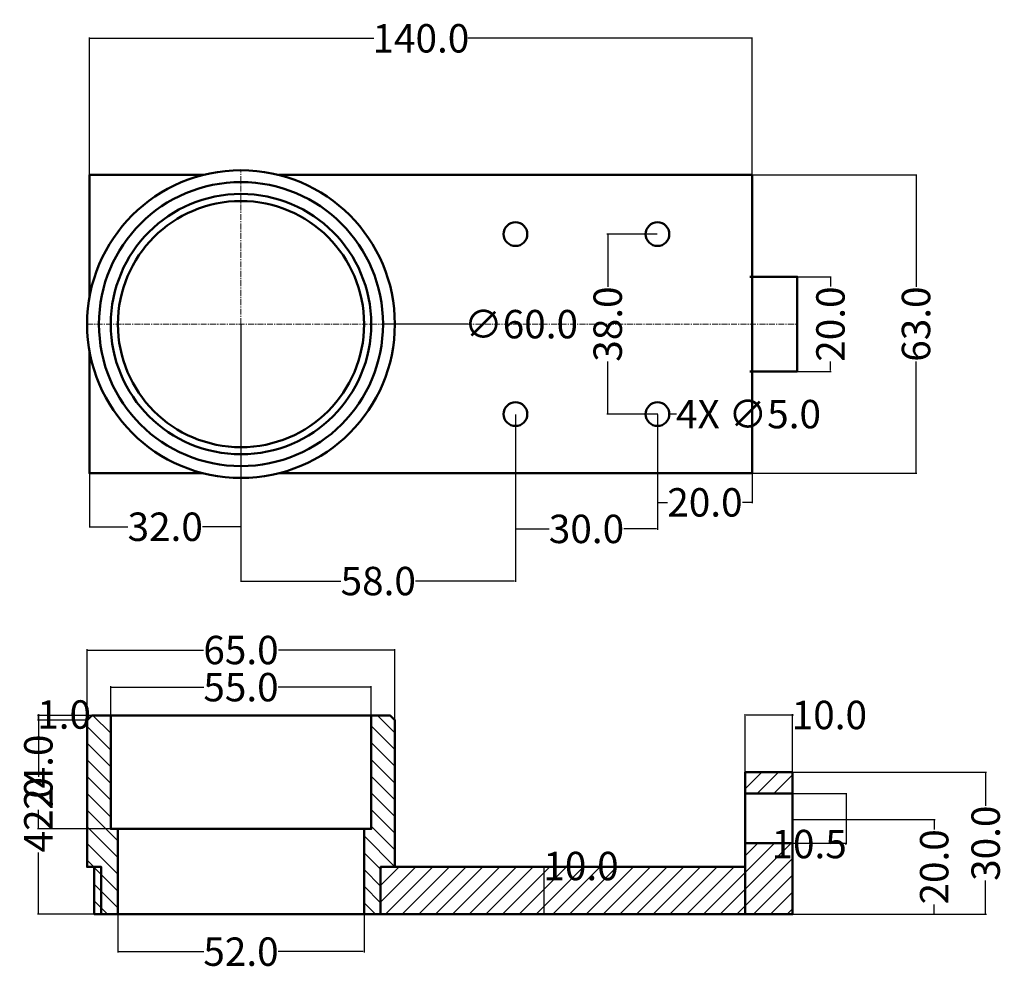
# Model space of a CAD drawing. Units: millimetres. Extents: x 92 to 300, y 40 to 241.
import ezdxf

# ---------------------------------------------------------------- set-up
doc = ezdxf.new("R2010")
doc.units = ezdxf.units.MM
doc.header["$MEASUREMENT"] = 0
doc.linetypes.add('CENTER', pattern=[2, 1.25, -0.25, 0.25, -0.25])
for name, color, linetype, lineweight in [('M-CNTR', 1, 'CENTER', 18), ('M-CONS', 8, 'Continuous', 13), ('M-DIMS', 2, 'Continuous', 25), ('M-HATC', 8, 'Continuous', 18), ('M-OUTL', 7, 'Continuous', 50), ('M-TEXT', 3, 'Continuous', 25)]:
    doc.layers.add(name, color=color, linetype=linetype, lineweight=lineweight)
doc.styles.get("Standard").update_dxf_attribs({"font": 'arial.ttf'})
doc.dimstyles.get("Standard").update_dxf_attribs({"dimtxt": 6, "dimasz": 0.18, "dimexe": 0.18, "dimexo": 0.0625, "dimgap": 0.09, "dimtad": 0, "dimtoh": 1, "dimdec": 1, "dimzin": 0, "dimdsep": 46, "dimtxsty": 'Standard', "dimcen": 0.09, "dimadec": 0, "dimazin": 0, "dimtfac": 1, "dimtdec": 1, "dimtofl": 0, "dimtmove": 0, "dimatfit": 3, "dimfxl": 1, "dimtolj": 1, "dimtzin": 0, "dimarcsym": 0})
pattern_1 = [(45, (89.012, 127.1657), (-1.767767, 1.767767), [])]

# ---------------------------------------------------------------- blocks, each defined once
blk = doc.blocks.new('*D1')
at = {"layer": 'Defpoints', "color": 0, "transparency": 16777216}
for p in [(247.12, 208.35), (247.12, 145.35), (281.69, 145.35)]:
    blk.add_point(p, dxfattribs=at)
at = {"layer": 'M-DIMS', "color": 0, "lineweight": -2, "transparency": 16777216}
for p, q in [((247.18, 208.35), (281.87, 208.35)), ((281.69, 208.17), (281.69, 184.73)), ((281.69, 145.53), (281.69, 168.96)), ((247.18, 145.35), (281.87, 145.35))]:
    blk.add_line(p, q, dxfattribs=at)
at = {"layer": 'M-DIMS', "color": 0, "transparency": 16777216}
for points in [[(281.66, 208.17), (281.72, 208.17), (281.69, 208.35)], [(281.66, 145.53), (281.72, 145.53), (281.69, 145.35)]]:
    blk.add_solid(points, dxfattribs=at)
at = {"layer": 'M-DIMS', "color": 0, "transparency": 16777216, "insert": (281.69, 176.85), "char_height": 6, "attachment_point": 5, "rotation": 90}
blk.add_mtext('\\A1;63.0', dxfattribs=at)
blk = doc.blocks.new('*D2')
at = {"layer": 'Defpoints', "color": 0, "transparency": 16777216}
for p in [(256.62, 186.85), (256.62, 166.85), (263.62, 166.85)]:
    blk.add_point(p, dxfattribs=at)
at = {"layer": 'M-DIMS', "color": 0, "lineweight": -2, "transparency": 16777216}
for p, q in [((256.68, 186.85), (263.8, 186.85)), ((263.62, 186.67), (263.62, 184.77)), ((263.62, 167.03), (263.62, 168.92)), ((256.68, 166.85), (263.8, 166.85))]:
    blk.add_line(p, q, dxfattribs=at)
at = {"layer": 'M-DIMS', "color": 0, "transparency": 16777216}
for points in [[(263.59, 186.67), (263.65, 186.67), (263.62, 186.85)], [(263.59, 167.03), (263.65, 167.03), (263.62, 166.85)]]:
    blk.add_solid(points, dxfattribs=at)
at = {"layer": 'M-DIMS', "color": 0, "transparency": 16777216, "insert": (263.62, 176.85), "char_height": 6, "attachment_point": 5, "rotation": 90}
blk.add_mtext('\\A1;20.0', dxfattribs=at)
blk = doc.blocks.new('*D3')
at = {"layer": 'Defpoints', "color": 0, "transparency": 16777216}
for p in [(227.09, 195.85), (216.57, 157.85), (227.09, 157.85)]:
    blk.add_point(p, dxfattribs=at)
at = {"layer": 'M-DIMS', "color": 0, "lineweight": -2, "transparency": 16777216}
for p, q in [((227.03, 195.85), (216.39, 195.85)), ((216.57, 195.67), (216.57, 184.72)), ((216.57, 158.03), (216.57, 168.97)), ((227.03, 157.85), (216.39, 157.85))]:
    blk.add_line(p, q, dxfattribs=at)
at = {"layer": 'M-DIMS', "color": 0, "transparency": 16777216}
for points in [[(216.54, 195.67), (216.6, 195.67), (216.57, 195.85)], [(216.54, 158.03), (216.6, 158.03), (216.57, 157.85)]]:
    blk.add_solid(points, dxfattribs=at)
at = {"layer": 'M-DIMS', "color": 0, "transparency": 16777216, "insert": (216.57, 176.85), "char_height": 6, "attachment_point": 5, "rotation": 90}
blk.add_mtext('\\A1;38.0', dxfattribs=at)
blk = doc.blocks.new('*D4')
at = {"layer": 'Defpoints', "color": 0, "transparency": 16777216}
for p in [(107.12, 145.35), (139.12, 144.35), (107.12, 134.05)]:
    blk.add_point(p, dxfattribs=at)
at = {"layer": 'M-DIMS', "color": 0, "lineweight": -2, "transparency": 16777216}
for p, q in [((107.12, 145.28), (107.12, 133.87)), ((139.12, 144.28), (139.12, 133.87)), ((107.3, 134.05), (115.25, 134.05)), ((138.94, 134.05), (130.99, 134.05))]:
    blk.add_line(p, q, dxfattribs=at)
at = {"layer": 'M-DIMS', "color": 0, "transparency": 16777216}
for points in [[(107.3, 134.08), (107.3, 134.02), (107.12, 134.05)], [(138.94, 134.08), (138.94, 134.02), (139.12, 134.05)]]:
    blk.add_solid(points, dxfattribs=at)
at = {"layer": 'M-DIMS', "color": 0, "transparency": 16777216, "insert": (123.12, 134.05), "char_height": 6, "attachment_point": 5}
blk.add_mtext('\\A1;32.0', dxfattribs=at)
blk = doc.blocks.new('*D5')
at = {"layer": 'Defpoints', "color": 0, "transparency": 16777216}
for p in [(247.12, 237.21), (107.12, 208.35), (247.12, 208.35)]:
    blk.add_point(p, dxfattribs=at)
at = {"layer": 'M-DIMS', "color": 0, "lineweight": -2, "transparency": 16777216}
for p, q in [((107.12, 208.41), (107.12, 237.39)), ((107.3, 237.21), (167.2, 237.21)), ((246.94, 237.21), (187.04, 237.21)), ((247.12, 208.41), (247.12, 237.39))]:
    blk.add_line(p, q, dxfattribs=at)
at = {"layer": 'M-DIMS', "color": 0, "transparency": 16777216}
for points in [[(107.3, 237.24), (107.3, 237.18), (107.12, 237.21)], [(246.94, 237.24), (246.94, 237.18), (247.12, 237.21)]]:
    blk.add_solid(points, dxfattribs=at)
at = {"layer": 'M-DIMS', "color": 0, "transparency": 16777216, "insert": (177.12, 237.21), "char_height": 6, "attachment_point": 5}
blk.add_mtext('\\A1;140.0', dxfattribs=at)
blk = doc.blocks.new('*D6')
at = {"layer": 'Defpoints', "color": 0, "transparency": 16777216}
for p in [(197.09, 157.85), (227.09, 157.85), (227.09, 133.59)]:
    blk.add_point(p, dxfattribs=at)
at = {"layer": 'M-DIMS', "color": 0, "lineweight": -2, "transparency": 16777216}
for p, q in [((197.09, 157.78), (197.09, 133.41)), ((227.09, 157.78), (227.09, 133.41)), ((197.27, 133.59), (204.22, 133.59)), ((226.91, 133.59), (219.96, 133.59))]:
    blk.add_line(p, q, dxfattribs=at)
at = {"layer": 'M-DIMS', "color": 0, "transparency": 16777216}
for points in [[(197.27, 133.62), (197.27, 133.56), (197.09, 133.59)], [(226.91, 133.62), (226.91, 133.56), (227.09, 133.59)]]:
    blk.add_solid(points, dxfattribs=at)
at = {"layer": 'M-DIMS', "color": 0, "transparency": 16777216, "insert": (212.09, 133.59), "char_height": 6, "attachment_point": 5}
blk.add_mtext('\\A1;30.0', dxfattribs=at)
blk = doc.blocks.new('*D7')
at = {"layer": 'Defpoints', "color": 0, "transparency": 16777216}
for p in [(227.09, 145.35), (247.12, 145.35), (247.12, 139.2)]:
    blk.add_point(p, dxfattribs=at)
at = {"layer": 'M-DIMS', "color": 0, "lineweight": -2, "transparency": 16777216}
for p, q in [((227.09, 145.28), (227.09, 139.02)), ((247.12, 145.28), (247.12, 139.02)), ((227.27, 139.2), (229.18, 139.2)), ((246.94, 139.2), (245.03, 139.2))]:
    blk.add_line(p, q, dxfattribs=at)
at = {"layer": 'M-DIMS', "color": 0, "transparency": 16777216}
for points in [[(227.27, 139.23), (227.27, 139.17), (227.09, 139.2)], [(246.94, 139.23), (246.94, 139.17), (247.12, 139.2)]]:
    blk.add_solid(points, dxfattribs=at)
at = {"layer": 'M-DIMS', "color": 0, "transparency": 16777216, "insert": (237.11, 139.2), "char_height": 6, "attachment_point": 5}
blk.add_mtext('\\A1;20.0', dxfattribs=at)
blk = doc.blocks.new('*D8')
at = {"layer": 'Defpoints', "color": 0, "transparency": 16777216}
for p in [(139.12, 176.85), (197.09, 157.85), (197.09, 122.58)]:
    blk.add_point(p, dxfattribs=at)
at = {"layer": 'M-DIMS', "color": 0, "lineweight": -2, "transparency": 16777216}
for p, q in [((139.12, 176.78), (139.12, 122.4)), ((197.09, 157.78), (197.09, 122.4)), ((139.3, 122.58), (160.23, 122.58)), ((196.91, 122.58), (175.98, 122.58))]:
    blk.add_line(p, q, dxfattribs=at)
at = {"layer": 'M-DIMS', "color": 0, "transparency": 16777216}
for points in [[(139.3, 122.61), (139.3, 122.55), (139.12, 122.58)], [(196.91, 122.61), (196.91, 122.55), (197.09, 122.58)]]:
    blk.add_solid(points, dxfattribs=at)
at = {"layer": 'M-DIMS', "color": 0, "transparency": 16777216, "insert": (168.11, 122.58), "char_height": 6, "attachment_point": 5}
blk.add_mtext('\\A1;58.0', dxfattribs=at)
blk = doc.blocks.new('*D9')
at = {"layer": 'Defpoints', "color": 0, "transparency": 16777216}
for p in [(255.62, 72.21), (285.53, 72.21), (255.62, 52.21)]:
    blk.add_point(p, dxfattribs=at)
at = {"layer": 'M-DIMS', "color": 0, "lineweight": -2, "transparency": 16777216}
for p, q in [((255.68, 72.21), (285.71, 72.21)), ((285.53, 72.03), (285.53, 70.13)), ((285.53, 52.39), (285.53, 54.29)), ((255.68, 52.21), (285.71, 52.21))]:
    blk.add_line(p, q, dxfattribs=at)
at = {"layer": 'M-DIMS', "color": 0, "transparency": 16777216}
for points in [[(285.5, 72.03), (285.56, 72.03), (285.53, 72.21)], [(285.5, 52.39), (285.56, 52.39), (285.53, 52.21)]]:
    blk.add_solid(points, dxfattribs=at)
at = {"layer": 'M-DIMS', "color": 0, "transparency": 16777216, "insert": (285.53, 62.21), "char_height": 6, "attachment_point": 5, "rotation": 90}
blk.add_mtext('\\A1;20.0', dxfattribs=at)
blk = doc.blocks.new('*D10')
at = {"layer": 'Defpoints', "color": 0, "transparency": 16777216}
for p in [(255.62, 94.29), (245.62, 82.21), (255.62, 82.21)]:
    blk.add_point(p, dxfattribs=at)
at = {"layer": 'M-DIMS', "color": 0, "lineweight": -2, "transparency": 16777216}
for p, q in [((245.62, 82.27), (245.62, 94.47)), ((245.8, 94.29), (255.44, 94.29)), ((255.62, 82.27), (255.62, 94.47)), ((255.62, 94.29), (255.8, 94.29))]:
    blk.add_line(p, q, dxfattribs=at)
at = {"layer": 'M-DIMS', "color": 0, "transparency": 16777216}
for points in [[(245.8, 94.32), (245.8, 94.26), (245.62, 94.29)], [(255.44, 94.32), (255.44, 94.26), (255.62, 94.29)]]:
    blk.add_solid(points, dxfattribs=at)
at = {"layer": 'M-DIMS', "color": 0, "transparency": 16777216, "insert": (263.39, 94.29), "char_height": 6, "attachment_point": 5}
blk.add_mtext('\\A1;10.0', dxfattribs=at)
blk = doc.blocks.new('*D11')
at = {"layer": 'Defpoints', "color": 0, "transparency": 16777216}
for p in [(166.62, 100.17), (111.62, 94.21), (166.62, 94.21)]:
    blk.add_point(p, dxfattribs=at)
at = {"layer": 'M-DIMS', "color": 0, "lineweight": -2, "transparency": 16777216}
for p, q in [((111.62, 94.27), (111.62, 100.35)), ((111.8, 100.17), (131.25, 100.17)), ((166.44, 100.17), (146.99, 100.17)), ((166.62, 94.27), (166.62, 100.35))]:
    blk.add_line(p, q, dxfattribs=at)
at = {"layer": 'M-DIMS', "color": 0, "transparency": 16777216}
for points in [[(111.8, 100.2), (111.8, 100.14), (111.62, 100.17)], [(166.44, 100.2), (166.44, 100.14), (166.62, 100.17)]]:
    blk.add_solid(points, dxfattribs=at)
at = {"layer": 'M-DIMS', "color": 0, "transparency": 16777216, "insert": (139.12, 100.17), "char_height": 6, "attachment_point": 5}
blk.add_mtext('\\A1;55.0', dxfattribs=at)
blk = doc.blocks.new('*D12')
at = {"layer": 'Defpoints', "color": 0, "transparency": 16777216}
for p in [(171.62, 108.01), (106.62, 93.21), (171.62, 93.21)]:
    blk.add_point(p, dxfattribs=at)
at = {"layer": 'M-DIMS', "color": 0, "lineweight": -2, "transparency": 16777216}
for p, q in [((106.62, 93.27), (106.62, 108.19)), ((171.62, 93.27), (171.62, 108.19)), ((106.8, 108.01), (131.23, 108.01)), ((171.44, 108.01), (147.01, 108.01))]:
    blk.add_line(p, q, dxfattribs=at)
at = {"layer": 'M-DIMS', "color": 0, "transparency": 16777216}
for points in [[(106.8, 108.04), (106.8, 107.98), (106.62, 108.01)], [(171.44, 108.04), (171.44, 107.98), (171.62, 108.01)]]:
    blk.add_solid(points, dxfattribs=at)
at = {"layer": 'M-DIMS', "color": 0, "transparency": 16777216, "insert": (139.12, 108.01), "char_height": 6, "attachment_point": 5}
blk.add_mtext('\\A1;65.0', dxfattribs=at)
blk = doc.blocks.new('*D13')
at = {"layer": 'Defpoints', "color": 0, "transparency": 16777216}
for p in [(113.12, 52.21), (165.12, 52.21), (165.12, 44.3)]:
    blk.add_point(p, dxfattribs=at)
at = {"layer": 'M-DIMS', "color": 0, "lineweight": -2, "transparency": 16777216}
for p, q in [((113.12, 52.15), (113.12, 44.12)), ((165.12, 52.15), (165.12, 44.12)), ((113.3, 44.3), (131.25, 44.3)), ((164.94, 44.3), (146.99, 44.3))]:
    blk.add_line(p, q, dxfattribs=at)
at = {"layer": 'M-DIMS', "color": 0, "transparency": 16777216}
for points in [[(113.3, 44.33), (113.3, 44.27), (113.12, 44.3)], [(164.94, 44.33), (164.94, 44.27), (165.12, 44.3)]]:
    blk.add_solid(points, dxfattribs=at)
at = {"layer": 'M-DIMS', "color": 0, "transparency": 16777216, "insert": (139.12, 44.3), "char_height": 6, "attachment_point": 5}
blk.add_mtext('\\A1;52.0', dxfattribs=at)
blk = doc.blocks.new('*D14')
at = {"layer": 'Defpoints', "color": 0, "transparency": 16777216}
for p in [(203.16, 62.21), (207.12, 62.21), (207.12, 52.21)]:
    blk.add_point(p, dxfattribs=at)
at = {"layer": 'M-DIMS', "color": 0, "lineweight": -2, "transparency": 16777216}
for p, q in [((203.16, 62.21), (203.16, 62.39)), ((203.16, 62.39), (203.34, 62.39)), ((207.06, 62.21), (202.98, 62.21)), ((203.16, 52.39), (203.16, 62.03)), ((207.06, 52.21), (202.98, 52.21))]:
    blk.add_line(p, q, dxfattribs=at)
at = {"layer": 'M-DIMS', "color": 0, "transparency": 16777216}
for points in [[(203.13, 62.03), (203.19, 62.03), (203.16, 62.21)], [(203.13, 52.39), (203.19, 52.39), (203.16, 52.21)]]:
    blk.add_solid(points, dxfattribs=at)
at = {"layer": 'M-DIMS', "color": 0, "transparency": 16777216, "insert": (210.93, 62.39), "char_height": 6, "attachment_point": 5}
blk.add_mtext('\\A1;10.0', dxfattribs=at)
blk = doc.blocks.new('*D15')
at = {"layer": 'Defpoints', "color": 0, "transparency": 16777216}
for p in [(250.62, 82.21), (250.62, 52.21), (296.4, 52.21)]:
    blk.add_point(p, dxfattribs=at)
at = {"layer": 'M-DIMS', "color": 0, "lineweight": -2, "transparency": 16777216}
for p, q in [((250.68, 82.21), (296.58, 82.21)), ((296.4, 82.03), (296.4, 75.08)), ((296.4, 52.39), (296.4, 59.34)), ((250.68, 52.21), (296.58, 52.21))]:
    blk.add_line(p, q, dxfattribs=at)
at = {"layer": 'M-DIMS', "color": 0, "transparency": 16777216}
for points in [[(296.37, 82.03), (296.43, 82.03), (296.4, 82.21)], [(296.37, 52.39), (296.43, 52.39), (296.4, 52.21)]]:
    blk.add_solid(points, dxfattribs=at)
at = {"layer": 'M-DIMS', "color": 0, "transparency": 16777216, "insert": (296.4, 67.21), "char_height": 6, "attachment_point": 5, "rotation": 90}
blk.add_mtext('\\A1;30.0', dxfattribs=at)
blk = doc.blocks.new('HOLE-M5')
blk.add_circle((2.5, 2.5), 2.5)
blk = doc.blocks.new('*D17')
at = {"layer": 'Defpoints', "color": 0, "transparency": 16777216}
for p in [(107.62, 94.21), (96.32, 52.21), (108.12, 52.21)]:
    blk.add_point(p, dxfattribs=at)
at = {"layer": 'M-DIMS', "color": 0, "lineweight": -2, "transparency": 16777216}
for p, q in [((107.56, 94.21), (96.14, 94.21)), ((96.32, 94.03), (96.32, 81.2)), ((96.32, 52.39), (96.32, 65.22)), ((108.06, 52.21), (96.14, 52.21))]:
    blk.add_line(p, q, dxfattribs=at)
at = {"layer": 'M-DIMS', "color": 0, "transparency": 16777216}
for points in [[(96.29, 94.03), (96.35, 94.03), (96.32, 94.21)], [(96.29, 52.39), (96.35, 52.39), (96.32, 52.21)]]:
    blk.add_solid(points, dxfattribs=at)
at = {"layer": 'M-DIMS', "color": 0, "transparency": 16777216, "insert": (96.32, 73.21), "char_height": 6, "attachment_point": 5, "rotation": 90}
blk.add_mtext('\\A1;42.0', dxfattribs=at)
blk = doc.blocks.new('*D18')
at = {"layer": 'Defpoints', "color": 0, "transparency": 16777216}
for p in [(111.62, 94.21), (96.32, 70.21), (111.62, 70.21)]:
    blk.add_point(p, dxfattribs=at)
at = {"layer": 'M-DIMS', "color": 0, "lineweight": -2, "transparency": 16777216}
for p, q in [((111.56, 94.21), (96.14, 94.21)), ((96.32, 94.03), (96.32, 90.13)), ((96.32, 70.39), (96.32, 74.29)), ((111.56, 70.21), (96.14, 70.21))]:
    blk.add_line(p, q, dxfattribs=at)
at = {"layer": 'M-DIMS', "color": 0, "transparency": 16777216}
for points in [[(96.29, 94.03), (96.35, 94.03), (96.32, 94.21)], [(96.29, 70.39), (96.35, 70.39), (96.32, 70.21)]]:
    blk.add_solid(points, dxfattribs=at)
at = {"layer": 'M-DIMS', "color": 0, "transparency": 16777216, "insert": (96.32, 82.21), "char_height": 6, "attachment_point": 5, "rotation": 90}
blk.add_mtext('\\A1;24.0', dxfattribs=at)
blk = doc.blocks.new('*D19')
at = {"layer": 'Defpoints', "color": 0, "transparency": 16777216}
for p in [(96.32, 94.21), (107.62, 94.21), (106.62, 93.21)]:
    blk.add_point(p, dxfattribs=at)
at = {"layer": 'M-DIMS', "color": 0, "lineweight": -2, "transparency": 16777216}
for p, q in [((107.56, 94.21), (96.14, 94.21)), ((96.32, 94.21), (96.32, 94.39)), ((96.32, 94.39), (96.5, 94.39)), ((96.32, 93.39), (96.32, 94.03)), ((106.56, 93.21), (96.14, 93.21))]:
    blk.add_line(p, q, dxfattribs=at)
at = {"layer": 'M-DIMS', "color": 0, "transparency": 16777216}
for points in [[(96.29, 94.03), (96.35, 94.03), (96.32, 94.21)], [(96.29, 93.39), (96.35, 93.39), (96.32, 93.21)]]:
    blk.add_solid(points, dxfattribs=at)
at = {"layer": 'M-DIMS', "color": 0, "transparency": 16777216, "insert": (101.76, 94.39), "char_height": 6, "attachment_point": 5}
blk.add_mtext('\\A1;1.0', dxfattribs=at)
blk = doc.blocks.new('*D20')
at = {"layer": 'Defpoints', "color": 0, "transparency": 16777216}
for p in [(255.62, 77.71), (255.62, 67.21), (266.92, 67.21)]:
    blk.add_point(p, dxfattribs=at)
at = {"layer": 'M-DIMS', "color": 0, "lineweight": -2, "transparency": 16777216}
for p, q in [((255.68, 77.71), (267.1, 77.71)), ((266.92, 77.53), (266.92, 67.39)), ((255.68, 67.21), (267.1, 67.21)), ((266.92, 67.03), (266.74, 67.03)), ((266.92, 67.21), (266.92, 67.03))]:
    blk.add_line(p, q, dxfattribs=at)
at = {"layer": 'M-DIMS', "color": 0, "transparency": 16777216}
for points in [[(266.89, 77.53), (266.95, 77.53), (266.92, 77.71)], [(266.89, 67.39), (266.95, 67.39), (266.92, 67.21)]]:
    blk.add_solid(points, dxfattribs=at)
at = {"layer": 'M-DIMS', "color": 0, "transparency": 16777216, "insert": (259.12, 67.03), "char_height": 6, "attachment_point": 5}
blk.add_mtext('\\A1;10.5', dxfattribs=at)
blk = doc.blocks.new('*D21')
at = {"layer": 'Defpoints', "color": 0, "transparency": 16777216}
for p in [(109.12, 176.85), (169.12, 176.84)]:
    blk.add_point(p, dxfattribs=at)
at = {"layer": 'M-DIMS', "color": 0, "lineweight": -2, "transparency": 16777216}
for p, q in [((139.03, 176.85), (139.21, 176.85)), ((139.12, 176.76), (139.12, 176.94)), ((187.12, 176.84), (169.3, 176.84))]:
    blk.add_line(p, q, dxfattribs=at)
at = {"layer": 'M-DIMS', "color": 0, "transparency": 16777216}
blk.add_solid([(169.3, 176.87), (169.3, 176.81), (169.12, 176.84)], dxfattribs=at)
at = {"layer": 'M-DIMS', "color": 0, "transparency": 16777216, "insert": (198.26, 176.84), "char_height": 6, "attachment_point": 5}
blk.add_mtext('\\A1;∅60.0', dxfattribs=at)
blk = doc.blocks.new('*D22')
at = {"layer": 'Defpoints', "color": 0, "transparency": 16777216}
for p in [(224.59, 157.85), (229.59, 157.84)]:
    blk.add_point(p, dxfattribs=at)
at = {"layer": 'M-DIMS', "color": 0, "lineweight": -2, "transparency": 16777216}
for p, q in [((227, 157.85), (227.18, 157.85)), ((227.09, 157.76), (227.09, 157.94)), ((231.09, 157.84), (229.77, 157.84))]:
    blk.add_line(p, q, dxfattribs=at)
at = {"layer": 'M-DIMS', "color": 0, "transparency": 16777216}
blk.add_solid([(229.77, 157.87), (229.77, 157.81), (229.59, 157.84)], dxfattribs=at)
at = {"layer": 'M-DIMS', "color": 0, "transparency": 16777216, "insert": (246.31, 157.84), "char_height": 6, "attachment_point": 5}
blk.add_mtext('\\A1;4X ∅5.0', dxfattribs=at)

msp = doc.modelspace()

# ---------------------------------------------------------------- hatches: boundary and pattern name
at = {"layer": 'M-HATC'}
h = msp.add_hatch(dxfattribs=at)
h.set_pattern_fill('ANSI31', color=256, scale=20, angle=90)
h.set_pattern_definition([(135, (89.012, 127.1657), (-1.767767, -1.767767), [])])
h.paths.add_polyline_path([(111.62, 94.21), (107.62, 94.21), (106.62, 93.21), (106.62, 62.21), (109.62, 62.21), (109.62, 52.21), (113.12, 52.21), (113.12, 70.21), (111.62, 70.21)])
h.paths.add_polyline_path([(171.62, 93.21), (170.62, 94.21), (166.62, 94.21), (166.62, 70.21), (165.12, 70.21), (165.12, 52.21), (168.62, 52.21), (168.62, 62.21), (171.62, 62.21)])
h.paths.add_polyline_path([(109.62, 62.21), (108.12, 62.21), (108.12, 52.21), (109.62, 52.21)], flags=17)
h = msp.add_hatch(dxfattribs=at)
h.set_pattern_fill('ANSI31', color=256, scale=20)
h.set_pattern_definition(pattern_1)
h.paths.add_polyline_path([(255.62, 77.71), (255.62, 82.21), (245.62, 82.21), (245.62, 77.71)])
h.paths.add_polyline_path([(245.62, 52.21), (255.62, 52.21), (255.62, 67.21), (245.62, 67.21), (245.62, 62.21)])
h = msp.add_hatch(dxfattribs=at)
h.set_pattern_fill('ANSI31', color=256, scale=20)
h.set_pattern_definition(pattern_1)
h.paths.add_polyline_path([(245.62, 52.21), (245.62, 62.21), (171.62, 62.21), (168.62, 62.21), (168.62, 52.21)])

# ---------------------------------------------------------------- linework, layer by layer
at = {"layer": 'M-CNTR'}
msp.add_line((108.2, 186.85), (108.12, 186.85), dxfattribs=at)
for points in [[(139.12, 144.35), (139.12, 150.85), (139.12, 202.85), (139.12, 209.35)], [(106.62, 176.85), (246.62, 176.85), (256.62, 176.85)]]:
    msp.add_lwpolyline(points, dxfattribs=at)
at = {"layer": 'M-CONS'}
msp.add_line((227.09, 145.35), (227.09, 157.85), dxfattribs=at)
at = {"layer": 'M-OUTL'}
for p, q in [((111.62, 94.21), (111.62, 70.21)), ((255.62, 77.71), (245.62, 77.71)), ((255.62, 67.21), (245.62, 67.21))]:
    msp.add_line(p, q, dxfattribs=at)
for points in [[(107.12, 182.52), (107.12, 208.35), (131.12, 208.35)], [(147.12, 145.35), (247.12, 145.35), (247.12, 208.35), (147.12, 208.35)], [(246.62, 186.85), (256.62, 186.85), (256.62, 166.85), (246.62, 166.85)], [(107.12, 171.17), (107.12, 145.35), (131.12, 145.35)], [(166.62, 94.21), (111.62, 94.21), (107.62, 94.21), (106.62, 93.21), (106.62, 62.21), (109.62, 62.21), (109.62, 52.21)], [(245.62, 62.21), (245.62, 52.21), (255.62, 52.21), (255.62, 82.21), (245.62, 82.21), (245.62, 62.21), (171.62, 62.21), (171.62, 93.21), (170.62, 94.21), (166.62, 94.21), (166.62, 70.21), (111.62, 70.21), (113.12, 70.21), (113.12, 52.21)], [(245.62, 52.21), (245.62, 52.21), (168.62, 52.21), (165.12, 52.21), (165.12, 70.21)], [(165.12, 52.21), (113.12, 52.21), (109.62, 52.21), (108.12, 52.21), (108.12, 62.21)], [(171.62, 62.21), (168.62, 62.21), (168.62, 52.21)]]:
    msp.add_lwpolyline(points, dxfattribs=at)
for radius in [32.5, 30, 27.5, 26]:
    msp.add_circle((139.12, 176.85), radius, dxfattribs=at)

# ---------------------------------------------------------------- block references
for p in [(194.59, 193.35), (224.59, 193.35), (194.59, 155.34), (224.59, 155.34)]:
    msp.add_blockref('HOLE-M5', p, dxfattribs=at)

# ---------------------------------------------------------------- texts
at = {"layer": 'M-TEXT'}
msp.add_attdef('M5', (199.57, 158.18), '', height=0.2, dxfattribs=at)

# ---------------------------------------------------------------- dimensions: what is measured, and where the dimension line sits
at = {"layer": 'M-DIMS'}
for base, p1, p2, picture, middle in [((247.12, 237.21), (107.12, 208.35), (247.12, 208.35), '*D5', (177.12, 237.21)), ((197.09, 122.58), (139.12, 176.85), (197.09, 157.85), '*D8', (168.11, 122.58)), ((227.09, 133.59), (197.09, 157.85), (227.09, 157.85), '*D6', (212.09, 133.59)), ((107.12, 134.05), (139.12, 144.35), (107.12, 145.35), '*D4', (123.12, 134.05)), ((247.12, 139.2), (227.09, 145.35), (247.12, 145.35), '*D7', (237.11, 139.2)), ((171.62, 108.01), (106.62, 93.21), (171.62, 93.21), '*D12', (139.12, 108.01)), ((166.62, 100.17), (111.62, 94.21), (166.62, 94.21), '*D11', (139.12, 100.17)), ((255.62, 94.29), (245.62, 82.21), (255.62, 82.21), '*D10', (263.39, 94.29)), ((165.12, 44.3), (113.12, 52.21), (165.12, 52.21), '*D13', (139.12, 44.3))]:
    dim = msp.add_linear_dim(base=base, p1=p1, p2=p2, dimstyle='Standard', override={"dimclrd": 0, "dimclre": 0, "dimclrt": 0}, dxfattribs=at)
    dim.commit()
    dim.dimension.update_dxf_attribs({"geometry": picture, "text_midpoint": middle})
for base, p1, p2, override, picture, middle in [((281.69, 145.35), (247.12, 208.35), (247.12, 145.35), {"dimclrd": 0, "dimclre": 0, "dimclrt": 0}, '*D1', (281.69, 176.85)), ((216.57, 157.85), (227.09, 195.85), (227.09, 157.85), {"dimclrd": 0, "dimclre": 0, "dimclrt": 0}, '*D3', (216.57, 176.85)), ((263.62, 166.85), (256.62, 186.85), (256.62, 166.85), {"dimclrd": 0, "dimclre": 0, "dimclrt": 0}, '*D2', (263.62, 176.85)), ((96.32, 94.21), (106.62, 93.21), (107.62, 94.21), {"dimdec": 1, "dimlfac": 1, "dimrnd": 0, "dimzin": 0, "dimdsep": 46, "dimlunit": 2}, '*D19', (101.76, 94.39)), ((96.32, 52.21), (107.62, 94.21), (108.12, 52.21), {"dimdec": 1, "dimlfac": 1, "dimrnd": 0, "dimzin": 0, "dimdsep": 46, "dimlunit": 2}, '*D17', (96.32, 73.21)), ((96.32, 70.21), (111.62, 94.21), (111.62, 70.21), {"dimdec": 1, "dimlfac": 1, "dimrnd": 0, "dimzin": 0, "dimdsep": 46, "dimlunit": 2}, '*D18', (96.32, 82.21)), ((296.4, 52.21), (250.62, 82.21), (250.62, 52.21), {"dimclrd": 0, "dimclre": 0, "dimclrt": 0}, '*D15', (296.4, 67.21)), ((266.92, 67.21), (255.62, 77.71), (255.62, 67.21), {"dimdec": 1, "dimlfac": 1, "dimrnd": 0, "dimzin": 0, "dimdsep": 46, "dimlunit": 2}, '*D20', (259.12, 67.03)), ((285.53, 72.21), (255.62, 52.21), (255.62, 72.21), {"dimclrd": 0, "dimclre": 0, "dimclrt": 0}, '*D9', (285.53, 62.21)), ((203.16, 62.21), (207.12, 52.21), (207.12, 62.21), {"dimclrd": 0, "dimclre": 0, "dimclrt": 0}, '*D14', (210.93, 62.39))]:
    dim = msp.add_linear_dim(base=base, p1=p1, p2=p2, angle=90, dimstyle='Standard', override=override, dxfattribs=at)
    dim.commit()
    dim.dimension.update_dxf_attribs({"geometry": picture, "text_midpoint": middle})
dim = msp.add_diameter_dim_2p(p1=(109.12, 176.85), p2=(169.12, 176.84), dimstyle='Standard', override={"dimdec": 1, "dimlfac": 1, "dimrnd": 0, "dimzin": 0, "dimdsep": 46, "dimlunit": 2}, dxfattribs=at)
dim.commit()
dim.dimension.update_dxf_attribs({"geometry": '*D21', "text_midpoint": (187.12, 176.84), "dimtype": 163})
dim = msp.add_diameter_dim_2p(p1=(224.59, 157.85), p2=(229.59, 157.84), text='4X <>', dimstyle='Standard', override={"dimdec": 1, "dimlfac": 1, "dimrnd": 0, "dimzin": 0, "dimdsep": 46, "dimlunit": 2}, dxfattribs=at)
dim.commit()
dim.dimension.update_dxf_attribs({"geometry": '*D22', "text_midpoint": (231.09, 157.84), "dimtype": 163})

doc.saveas('drawing.dxf')
